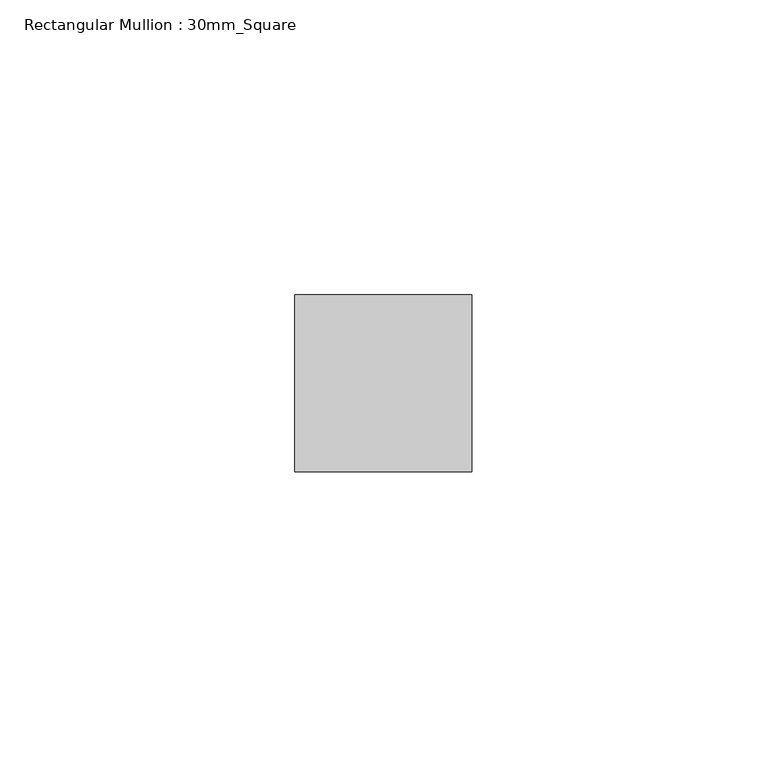
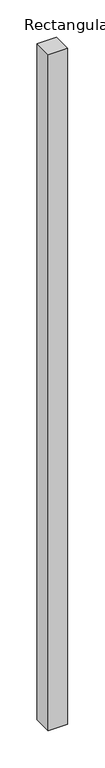
"""IFC4 building model written with IfcOpenShell, lengths in millimetres: member geometry, Rectangular Mullion : 30mm_Square."""

from ifc_helpers import new_model, si_unit, frame, origin, place, context, project, spatial, polyline, outline, extrude, source, transform, mapped, element, save


def rectangular_mullion_30mm_square_c90eb03c(model_context):
    return source(origin(), model_context, "Body", "SweptSolid", [
        extrude(outline(polyline([(0.0, 15.0), (0.0, -15.0), (-30.0, -15.0), (-30.0, 15.0), (0.0, 15.0)])), frame((0.0, 0.0, -1106.4666668), z_axis=(0.0, 0.0, 1.0), x_axis=(1.0, 0.0, 0.0)), (0.0, 0.0, 1.0), 1106.4666668),
    ])


if __name__ == "__main__":
    model = new_model("IFC4")
    model_context = context("Model", 3, world=origin())
    ifc_project = project(units=[si_unit("LENGTHUNIT", "METRE", prefix="MILLI")], contexts=[model_context])
    site = spatial("IfcSite", under=ifc_project)
    building = spatial("IfcBuilding", under=site)
    placement = place(None, origin())
    rectangular_mullion_30mm_square_shape = rectangular_mullion_30mm_square_c90eb03c(model_context)
    element("IfcMember", 1, ObjectType="Rectangular Mullion : 30mm_Square", at=placement, inside=building, context=model_context, shape_type="MappedRepresentation", body=[
        mapped(rectangular_mullion_30mm_square_shape, transform((0.0, 0.0, 0.0), x_axis=(1.0, 0.0, 0.0), y_axis=(0.0, 1.0, 0.0), z_axis=(0.0, 0.0, 1.0))),
    ])
    save(model, "model.ifc")

# Revit data of these elements
# Type "Rectangular Mullion : 30mm_Square"
#   Keynote = "H11"
#   built-in parameter 1007304 = 0.0984252 (stored number, unit not read)
#   built-in parameter 1007301 = 0.0492126 (stored number, unit not read)
#   built-in parameter 1007300 = 0.0492126 (stored number, unit not read)
# Element 1 (IfcMember, "Rectangular Mullion : 30mm_Square")
#   Materials on its faces: "Aluminium"
# Materials
#   "Aluminium": class "Metal", colour RGB 247 247 247, transparency 0, Description = "Aluminium 6061", Cost = 0
